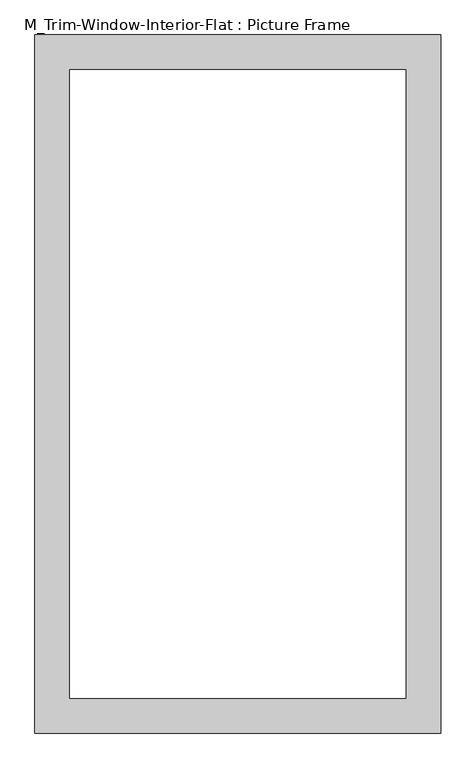
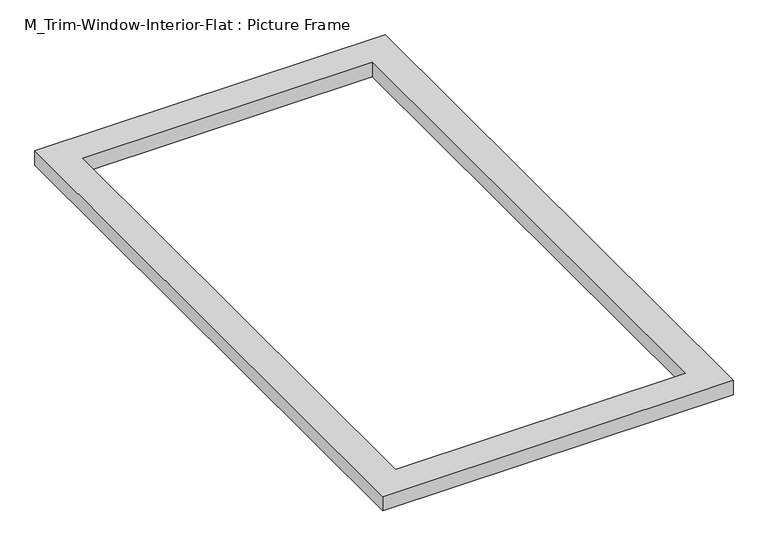
"""IFC4 building model written with IfcOpenShell, lengths in millimetres: proxy geometry, M_Trim-Window-Interior-Flat : Picture Frame."""

from ifc_helpers import new_model, si_unit, origin, origin_with_axes, place, context, project, spatial, polyline, outline, extrude, source, transform, mapped, element, save


def m_trim_window_interior_flat_picture_frame_87adca9b(model_context):
    return source(origin(), model_context, "Body", "SweptSolid", [
        extrude(outline(polyline([(347.3, 47.3), (347.3, -1147.3), (-347.3, -1147.3), (-347.3, 47.3), (347.3, 47.3)]), holes=[polyline([(287.3, -12.7), (-287.3, -12.7), (-287.3, -1087.3), (287.3, -1087.3), (287.3, -12.7)])]), origin_with_axes(), (0.0, 0.0, 1.0), 30.0),
    ])


if __name__ == "__main__":
    model = new_model("IFC4")
    model_context = context("Model", 3, world=origin())
    ifc_project = project(units=[si_unit("LENGTHUNIT", "METRE", prefix="MILLI")], contexts=[model_context])
    site = spatial("IfcSite", under=ifc_project)
    building = spatial("IfcBuilding", under=site)
    placement = place(None, origin())
    m_trim_window_interior_flat_picture_frame_shape = m_trim_window_interior_flat_picture_frame_87adca9b(model_context)
    element("IfcBuildingElementProxy", 1, Name="M_Trim-Window-Interior-Flat : Picture Frame", ObjectType="M_Trim-Window-Interior-Flat : Picture Frame", at=placement, inside=building, context=model_context, shape_type="MappedRepresentation", body=[
        mapped(m_trim_window_interior_flat_picture_frame_shape, transform((0.0, 0.0, 0.0), x_axis=(1.0, 0.0, 0.0), y_axis=(0.0, 1.0, 0.0), z_axis=(0.0, 0.0, 1.0))),
    ])
    save(model, "model.ifc")

# Revit data of these elements
# Type "M_Trim-Window-Interior-Flat : Picture Frame"
#   Trim Thickness_Picture Frame = 0.03 m
#   Trim Width = 0.06 m
#   Trim Thickness_with Sill = 0.02 m
#   Sill Thickness = 0.03 m
#   Opening Width [instance default] = 0.6 m
#   Opening Height [instance default] = 0.9 m
#   Default Elevation = 1.2 m
#   Sill = no
#   Picture Frame = yes
#   Trim Material [instance default] = none
# Element 1 (IfcBuildingElementProxy, "M_Trim-Window-Interior-Flat : Picture Frame")
#   Opening Height = 1.1 m
#   Trim Material = Wood - Stained
#   Materials on its faces: "Wood - Stained"
# Materials
#   "Wood - Stained": class "Wood", colour RGB 224 178 126, transparency 0, Cost = 0
